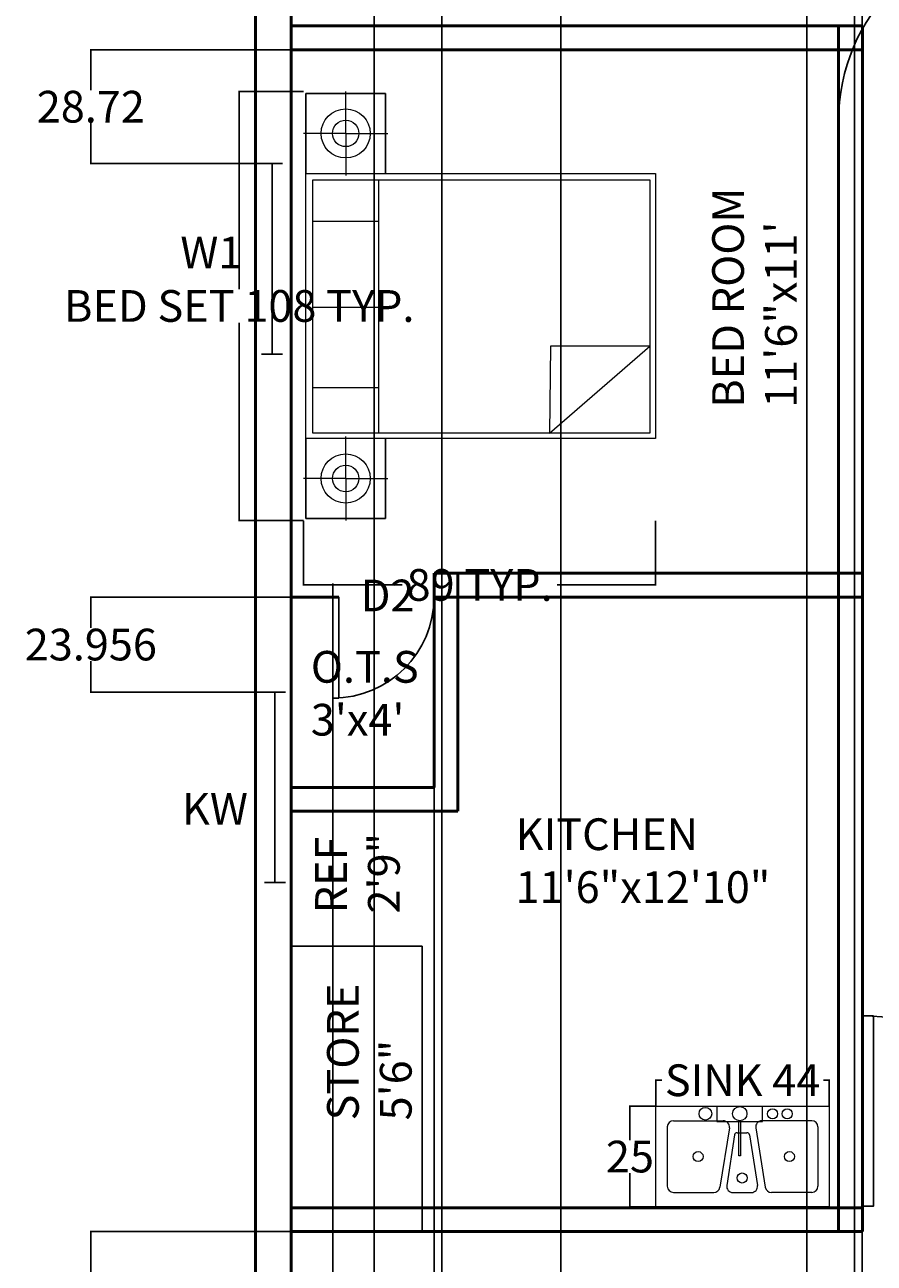
# Model space of a CAD drawing. Units: inches. Extents: x 3004 to 3478, y -798 to 114.
# Tile 3 of 5: x 3004 to 3218, y -503 to -190. Entities that reach past the tile are written whole.
import ezdxf

# ---------------------------------------------------------------- set-up
doc = ezdxf.new("R2010")
doc.units = ezdxf.units.IN
doc.header["$MEASUREMENT"] = 0
for name, color, linetype, lineweight in [('A-ANNO-DIMS', 2, 'Continuous', 18), ('A-ANNO-TEXT', 7, 'Continuous', 18), ('A-AREA-IDEN', 7, 'Continuous', 18), ('A-DOOR', 4, 'Continuous', 25), ('A-FLOR-CASE', 8, 'Continuous', 25), ('A-FLOR-FIXT', 9, 'Continuous', 18), ('A-FURN', 8, 'Continuous', 18), ('A-GLAZ', 4, 'Continuous', 25), ('A-WALL', 7, 'Continuous', 50)]:
    doc.layers.add(name, color=color, linetype=linetype, lineweight=lineweight)
doc.styles.get("Standard").update_dxf_attribs({"font": 'arial.ttf', "height": 8})
doc.dimstyles.get("Standard").update_dxf_attribs({"dimtxt": 0.18, "dimasz": 0.18, "dimexe": 0.18, "dimexo": 0.0625, "dimgap": 0.09, "dimtad": 0, "dimtih": 1, "dimtoh": 1, "dimzin": 0, "dimdsep": 46, "dimlunit": 4, "dimtxsty": 'Standard', "dimcen": 0.09, "dimadec": 0, "dimazin": 0, "dimtfac": 1, "dimtofl": 0, "dimtmove": 0, "dimatfit": 3, "dimfxl": 1, "dimtolj": 1, "dimtzin": 0, "dimarcsym": 0})

# ---------------------------------------------------------------- blocks, each defined once
blk = doc.blocks.new('A$C27EB6A15')
for p, q in [((0, 0), (0, 644.7)), ((0, 644.7), (1110.1, 644.7)), ((682.1, 643.4), (390.6, 643.4)), ((390.6, 643.4), (390.6, 547.6)), ((682.1, 547.6), (682.1, 643.4)), ((1110.1, 644.7), (1110.1, 0)), ((72.5, 512.3), (72.5, 132)), ((111.7, 551.5), (431.6, 551.5)), ((390.6, 547.6), (682.1, 547.6)), ((470.2, 506.2), (409.5, 125.9)), ((530.7, 328), (530.7, 553.3)), ((541.9, 552.9), (541.9, 328)), ((639.9, 506.2), (700.6, 125.9)), ((998.4, 551.5), (678.5, 551.5)), ((1037.5, 512.3), (1037.5, 132)), ((504.1, 462.2), (453.4, 137.6)), ((519.5, 475.4), (583.2, 475.4)), ((598.6, 462.2), (650.4, 137.8)), ((541.9, 328), (530.7, 328)), ((111.7, 92.9), (370.9, 92.9)), ((492.1, 92.5), (611.7, 92.5)), ((998.4, 92.9), (739.2, 92.9)), ((1110.1, 0), (0, 0))]:
    blk.add_line(p, q)
for centre, radius in [((317, 596.6), 40.3), ((537.2, 597.3), 45.9), ((747.1, 596.6), 32.3), ((841.3, 596.6), 32.3), ((269.9, 322.4), 32.3), ((854.7, 322.4), 32.3), ((552.2, 185.3), 32.3)]:
    blk.add_circle(centre, radius)
for centre, radius, start, end in [((111.7, 512.3), 39.1, 90, 180), ((431.6, 512.3), 39.1, 350.93428, 90), ((538.2, 591.7), 39.2, 259.3674, 275.24456), ((678.5, 512.3), 39.1, 90, 189.06572), ((998.4, 512.3), 39.1, 0, 90), ((519.5, 459.7), 15.7, 90, 171.13117), ((583.2, 459.7), 15.7, 9.06572, 90), ((111.7, 132), 39.1, 180, 270), ((370.9, 132), 39.1, 270, 350.93428), ((492.1, 131.6), 39.1, 171.13117, 270), ((611.7, 131.6), 39.1, 270, 9.06572), ((739.2, 132), 39.1, 189.06572, 270), ((998.4, 132), 39.1, 270, 0)]:
    blk.add_arc(centre, radius, start, end)
blk = doc.blocks.new('A$C214F6537')
for p, q in [((0.4648, 1.98, -0.1688), (0.0108, 1.98, -0.1688)), ((0.0108, 1.98, -0.1688), (0.0108, 1.53, -0.1688)), ((0.0108, 1.98, -0.1688), (2.4188, 1.98, -0.1688)), ((0.0108, 1.53, -0.1688), (0.0108, 1.98, -0.1688)), ((0.2381, 1.7553, -0.4388), (0.2381, 1.9934, -0.4388)), ((0.4648, 0, -0.1688), (0.4648, 1.98, -0.1688)), ((0.4648, 1.98, -0.1688), (1.9648, 1.98, -0.1688)), ((0.4648, 1.53, -0.1688), (0.4648, 1.98, -0.1688)), ((1.9648, 1.98, -0.1688), (1.9648, 0, -0.1688)), ((2.4188, 1.98, -0.1688), (1.9648, 1.98, -0.1688)), ((1.9648, 1.98, -0.1688), (1.9648, 1.53, -0.1688)), ((2.1921, 1.7553, -0.4388), (2.1921, 1.9934, -0.4388)), ((2.4188, 1.53, -0.1688), (2.4188, 1.98, -0.1688)), ((2.4188, 1.98, -0.1688), (2.4188, 1.53, -0.1688)), ((0.4951, 1.9415, -0.1688), (1.9289, 1.9415, -0.1688)), ((0.4951, 1.5702, -0.1688), (0.4951, 1.9415, -0.1688)), ((0.7525, 1.9415, -0.1688), (0.7525, 1.5702, -0.1688)), ((1.2089, 1.9415, -0.1688), (1.2089, 1.5702, -0.1688)), ((1.6942, 1.9415, -0.1688), (1.6942, 1.5702, -0.1688)), ((1.9289, 1.9415, -0.1688), (1.9289, 1.5702, -0.1688)), ((0.2381, 1.7553, -0.4388), (0, 1.7553, -0.4388)), ((0.2381, 1.7553, -0.4388), (0.2381, 1.5173, -0.4388)), ((0.2381, 1.7553, -0.4388), (0.4762, 1.7553, -0.4388)), ((2.1921, 1.7553, -0.4388), (1.954, 1.7553, -0.4388)), ((2.1921, 1.7553, -0.4388), (2.4302, 1.7553, -0.4388)), ((2.1921, 1.7553, -0.4388), (2.1921, 1.5173, -0.4388)), ((0.4951, 0.0322, -0.1688), (0.4951, 1.5702, -0.1688)), ((1.9289, 1.5702, -0.1688), (0.4951, 1.5702, -0.1688)), ((1.9289, 1.5702, -0.1688), (1.9289, 0.0322, -0.1688)), ((0.0108, 1.53, -0.1688), (0.4648, 1.53, -0.1688)), ((0.4648, 1.53, -0.1688), (0.0108, 1.53, -0.1688)), ((0.4648, 0, -0.1688), (0.4648, 1.53, -0.1688)), ((1.9648, 1.53, -0.1688), (2.4188, 1.53, -0.1688)), ((2.4188, 1.53, -0.1688), (1.9648, 1.53, -0.1688)), ((1.9648, 1.53, -0.1688), (1.9648, 0, -0.1688)), ((0.4951, 0.6005, -0.1688), (0.9872, 0.0322, -0.1688)), ((0.9872, 0.5947, -0.1688), (0.4951, 0.6005, -0.1688)), ((0.9872, 0.0322, -0.1688), (0.9872, 0.5947, -0.1688)), ((1.9648, 0, -0.1688), (0.4648, 0, -0.1688)), ((1.9648, 0, -0.1688), (0.4648, 0, -0.1688)), ((1.9289, 0.0322, -0.1688), (0.4951, 0.0322, -0.1688))]:
    blk.add_line(p, q)
for centre, radius in [((0.2381, 1.7553, -0.4388), 0.139), ((2.1921, 1.7553, -0.4388), 0.139), ((0.2381, 1.7553, -0.4388), 0.075), ((2.1921, 1.7553, -0.4388), 0.075)]:
    blk.add_circle(centre, radius)
blk = doc.blocks.new('*U17')
for p, q in [((-750, 0), (-750, -100)), ((0, 0), (0, -100))]:
    blk.add_line(p, q)
blk.add_lwpolyline([(0, 0), (0, 750), (-43.75, 750), (-43.75, 0)], close=True)
blk.add_arc((0, 0), 750, 90, 180)
blk = doc.blocks.new('*U18')
for p, q in [((0, 0), (0, 100)), ((750, 0), (750, 100))]:
    blk.add_line(p, q)
blk.add_lwpolyline([(0, 0), (0, -750), (43.75, -750), (43.75, 0)], close=True)
blk.add_arc((0, 0), 750, 270, 0)
blk = doc.blocks.new('*U16')
for p, q in [((0, 0), (0, -100)), ((750, 0), (750, -100))]:
    blk.add_line(p, q)
blk.add_lwpolyline([(0, 0), (0, 750), (43.75, 750), (43.75, 0)], close=True)
blk.add_arc((0, 0), 750, 0, 90)
blk = doc.blocks.new('Window - Imperial')
for p, q in [((0, 4), (0, 0)), ((36, 4), (36, 0)), ((0, 2), (36, 2))]:
    blk.add_line(p, q)
blk = doc.blocks.new('*D24')
at = {"layer": 'A-ANNO-DIMS', "color": 0, "lineweight": -2, "transparency": 16777216}
for p, q in [((3074.26, -207.17), (3057.91, -207.17)), ((3058.09, -207.35), (3058.09, -257.05)), ((3058.09, -315.21), (3058.09, -265.5)), ((3074.26, -315.39), (3057.91, -315.39))]:
    blk.add_line(p, q, dxfattribs=at)
at = {"layer": 'A-ANNO-DIMS', "color": 0, "transparency": 16777216}
for points in [[(3058.06, -207.35), (3058.12, -207.35), (3058.09, -207.17)], [(3058.06, -315.21), (3058.12, -315.21), (3058.09, -315.39)]]:
    blk.add_solid(points, dxfattribs=at)
at = {"layer": 'Defpoints', "color": 0, "transparency": 16777216}
for p in [(3058.09, -207.17), (3074.32, -207.17), (3074.32, -315.39)]:
    blk.add_point(p, dxfattribs=at)
at = {"layer": 'A-ANNO-DIMS', "color": 0, "transparency": 16777216, "insert": (3058.09, -261.28), "char_height": 8, "attachment_point": 5}
blk.add_mtext('\\A1;BED SET 108 TYP.', dxfattribs=at)
blk = doc.blocks.new('*D25')
at = {"layer": 'A-ANNO-DIMS', "color": 0, "lineweight": -2, "transparency": 16777216}
for p, q in [((3074.32, -315.45), (3074.32, -331.8)), ((3163.09, -315.45), (3163.09, -331.8)), ((3074.5, -331.62), (3099.14, -331.62)), ((3162.91, -331.62), (3138.27, -331.62))]:
    blk.add_line(p, q, dxfattribs=at)
at = {"layer": 'A-ANNO-DIMS', "color": 0, "transparency": 16777216}
for points in [[(3074.5, -331.59), (3074.5, -331.65), (3074.32, -331.62)], [(3162.91, -331.59), (3162.91, -331.65), (3163.09, -331.62)]]:
    blk.add_solid(points, dxfattribs=at)
at = {"layer": 'Defpoints', "color": 0, "transparency": 16777216}
for p in [(3074.32, -315.39), (3163.09, -315.39), (3074.32, -331.62)]:
    blk.add_point(p, dxfattribs=at)
at = {"layer": 'A-ANNO-DIMS', "color": 0, "transparency": 16777216, "insert": (3118.7, -331.62), "char_height": 8, "attachment_point": 5}
blk.add_mtext('\\A1;89 TYP.', dxfattribs=at)
blk = doc.blocks.new('*D30')
at = {"layer": 'A-ANNO-DIMS', "color": 0, "lineweight": -2, "transparency": 16777216}
for p, q in [((3163.16, -463.02), (3163.16, -456.34)), ((3163.34, -456.52), (3164.64, -456.52)), ((3206.69, -456.52), (3205.4, -456.52)), ((3206.87, -463.02), (3206.87, -456.34))]:
    blk.add_line(p, q, dxfattribs=at)
at = {"layer": 'A-ANNO-DIMS', "color": 0, "transparency": 16777216}
for points in [[(3163.34, -456.49), (3163.34, -456.55), (3163.16, -456.52)], [(3206.69, -456.49), (3206.69, -456.55), (3206.87, -456.52)]]:
    blk.add_solid(points, dxfattribs=at)
at = {"layer": 'Defpoints', "color": 0, "transparency": 16777216}
for p in [(3206.87, -456.52), (3163.16, -463.08), (3206.87, -463.08)]:
    blk.add_point(p, dxfattribs=at)
at = {"layer": 'A-ANNO-DIMS', "color": 0, "transparency": 16777216, "insert": (3185.02, -456.52), "char_height": 8, "attachment_point": 5}
blk.add_mtext('\\A1;SINK 44', dxfattribs=at)
blk = doc.blocks.new('*D31')
at = {"layer": 'A-ANNO-DIMS', "color": 0, "lineweight": -2, "transparency": 16777216}
for p, q in [((3163.1, -463.08), (3156.43, -463.08)), ((3156.61, -463.26), (3156.61, -471.6)), ((3156.61, -488.28), (3156.61, -479.95)), ((3163.1, -488.46), (3156.43, -488.46))]:
    blk.add_line(p, q, dxfattribs=at)
at = {"layer": 'A-ANNO-DIMS', "color": 0, "transparency": 16777216}
for points in [[(3156.58, -463.26), (3156.64, -463.26), (3156.61, -463.08)], [(3156.58, -488.28), (3156.64, -488.28), (3156.61, -488.46)]]:
    blk.add_solid(points, dxfattribs=at)
at = {"layer": 'Defpoints', "color": 0, "transparency": 16777216}
for p in [(3156.61, -463.08), (3163.16, -463.08), (3163.16, -488.46)]:
    blk.add_point(p, dxfattribs=at)
at = {"layer": 'A-ANNO-DIMS', "color": 0, "transparency": 16777216, "insert": (3156.61, -475.77), "char_height": 8, "attachment_point": 5}
blk.add_mtext('\\A1;25', dxfattribs=at)
blk = doc.blocks.new('*D50')
at = {"layer": 'A-ANNO-DIMS', "color": 0, "lineweight": -2, "transparency": 16777216}
for p, q in [((3071.15, -196.68), (3020.48, -196.68)), ((3020.66, -196.86), (3020.66, -206.86)), ((3020.66, -225.22), (3020.66, -215.21)), ((3063.64, -225.4), (3020.48, -225.4))]:
    blk.add_line(p, q, dxfattribs=at)
at = {"layer": 'A-ANNO-DIMS', "color": 0, "transparency": 16777216}
for points in [[(3020.63, -196.86), (3020.69, -196.86), (3020.66, -196.68)], [(3020.63, -225.22), (3020.69, -225.22), (3020.66, -225.4)]]:
    blk.add_solid(points, dxfattribs=at)
at = {"layer": 'Defpoints', "color": 0, "transparency": 16777216}
for p in [(3071.21, -196.68), (3020.66, -225.4), (3063.7, -225.4)]:
    blk.add_point(p, dxfattribs=at)
at = {"layer": 'A-ANNO-DIMS', "color": 0, "transparency": 16777216, "insert": (3020.66, -211.04), "char_height": 8, "attachment_point": 5}
blk.add_mtext('\\A1;28.72', dxfattribs=at)
blk = doc.blocks.new('*D51')
at = {"layer": 'A-ANNO-DIMS', "color": 0, "lineweight": -2, "transparency": 16777216}
for p, q in [((3071.15, -334.68), (3020.48, -334.68)), ((3020.66, -334.86), (3020.66, -342.48)), ((3020.66, -358.45), (3020.66, -350.83)), ((3064.37, -358.63), (3020.48, -358.63))]:
    blk.add_line(p, q, dxfattribs=at)
at = {"layer": 'A-ANNO-DIMS', "color": 0, "transparency": 16777216}
for points in [[(3020.63, -334.86), (3020.69, -334.86), (3020.66, -334.68)], [(3020.63, -358.45), (3020.69, -358.45), (3020.66, -358.63)]]:
    blk.add_solid(points, dxfattribs=at)
at = {"layer": 'Defpoints', "color": 0, "transparency": 16777216}
for p in [(3071.21, -334.68), (3020.66, -358.63), (3064.43, -358.63)]:
    blk.add_point(p, dxfattribs=at)
at = {"layer": 'A-ANNO-DIMS', "color": 0, "transparency": 16777216, "insert": (3020.66, -346.66), "char_height": 8, "attachment_point": 5}
blk.add_mtext('\\A1;23.956', dxfattribs=at)
blk = doc.blocks.new('*D52')
at = {"layer": 'A-ANNO-DIMS', "color": 0, "lineweight": -2, "transparency": 16777216}
for p, q in [((3071.15, -494.68), (3020.48, -494.68)), ((3020.66, -494.86), (3020.66, -517.2)), ((3020.66, -547.9), (3020.66, -525.56)), ((3064.06, -548.08), (3020.48, -548.08))]:
    blk.add_line(p, q, dxfattribs=at)
at = {"layer": 'A-ANNO-DIMS', "color": 0, "transparency": 16777216}
for points in [[(3020.63, -494.86), (3020.69, -494.86), (3020.66, -494.68)], [(3020.63, -547.9), (3020.69, -547.9), (3020.66, -548.08)]]:
    blk.add_solid(points, dxfattribs=at)
at = {"layer": 'Defpoints', "color": 0, "transparency": 16777216}
for p in [(3071.21, -494.68), (3020.66, -548.08), (3064.12, -548.08)]:
    blk.add_point(p, dxfattribs=at)
at = {"layer": 'A-ANNO-DIMS', "color": 0, "transparency": 16777216, "insert": (3020.66, -521.38), "char_height": 8, "attachment_point": 5}
blk.add_mtext('\\A1;53.4', dxfattribs=at)
blk = doc.blocks.new('*D53')
at = {"layer": 'A-ANNO-DIMS', "color": 0, "lineweight": -2, "transparency": 16777216}
for p, q in [((3092.13, 11.22), (3092.13, -793.41)), ((3071.21, 7.26), (3071.21, -793.41)), ((3071.39, -793.23), (3091.95, -793.23)), ((3092.13, -793.23), (3092.31, -793.23))]:
    blk.add_line(p, q, dxfattribs=at)
at = {"layer": 'A-ANNO-DIMS', "color": 0, "transparency": 16777216}
for points in [[(3071.39, -793.2), (3071.39, -793.26), (3071.21, -793.23)], [(3091.95, -793.2), (3091.95, -793.26), (3092.13, -793.23)]]:
    blk.add_solid(points, dxfattribs=at)
at = {"layer": 'Defpoints', "color": 0, "transparency": 16777216}
for p in [(3092.13, 11.28), (3071.21, 7.32), (3092.13, -793.23)]:
    blk.add_point(p, dxfattribs=at)
at = {"layer": 'A-ANNO-DIMS', "color": 0, "transparency": 16777216, "insert": (3105.93, -793.23), "char_height": 8, "attachment_point": 5}
blk.add_mtext('\\A1;20.92', dxfattribs=at)
blk = doc.blocks.new('*D55')
at = {"layer": 'A-ANNO-DIMS', "color": 0, "lineweight": -2, "transparency": 16777216}
for p, q in [((3215.21, -494.62), (3215.21, 109.05)), ((3215.39, 108.87), (3233.22, 108.87)), ((3263.03, 108.87), (3245.2, 108.87)), ((3263.21, -494.62), (3263.21, 109.05))]:
    blk.add_line(p, q, dxfattribs=at)
at = {"layer": 'A-ANNO-DIMS', "color": 0, "transparency": 16777216}
for points in [[(3215.39, 108.9), (3215.39, 108.84), (3215.21, 108.87)], [(3263.03, 108.9), (3263.03, 108.84), (3263.21, 108.87)]]:
    blk.add_solid(points, dxfattribs=at)
at = {"layer": 'Defpoints', "color": 0, "transparency": 16777216}
for p in [(3263.21, 108.87), (3215.21, -494.68), (3263.21, -494.68)]:
    blk.add_point(p, dxfattribs=at)
at = {"layer": 'A-ANNO-DIMS', "color": 0, "transparency": 16777216, "insert": (3239.21, 108.87), "char_height": 8, "attachment_point": 5}
blk.add_mtext('\\A1;48', dxfattribs=at)
blk = doc.blocks.new('*D57')
at = {"layer": 'A-ANNO-DIMS', "color": 0, "lineweight": -2, "transparency": 16777216}
for p, q in [((3201.21, -644.62), (3201.21, 109.05)), ((3201.39, 108.87), (3201.81, 108.87)), ((3213.03, 108.87), (3212.61, 108.87)), ((3213.21, -644.62), (3213.21, 109.05))]:
    blk.add_line(p, q, dxfattribs=at)
at = {"layer": 'A-ANNO-DIMS', "color": 0, "transparency": 16777216}
for points in [[(3201.39, 108.9), (3201.39, 108.84), (3201.21, 108.87)], [(3213.03, 108.9), (3213.03, 108.84), (3213.21, 108.87)]]:
    blk.add_solid(points, dxfattribs=at)
at = {"layer": 'Defpoints', "color": 0, "transparency": 16777216}
for p in [(3213.21, 108.87), (3201.21, -644.68), (3213.21, -644.68)]:
    blk.add_point(p, dxfattribs=at)
at = {"layer": 'A-ANNO-DIMS', "color": 0, "transparency": 16777216, "insert": (3207.21, 108.87), "char_height": 8, "attachment_point": 5}
blk.add_mtext('\\A1;12', dxfattribs=at)
blk = doc.blocks.new('*D62')
at = {"layer": 'A-ANNO-DIMS', "color": 0, "lineweight": -2, "transparency": 16777216}
for p, q in [((3081.71, -334.74), (3081.71, -793.41)), ((3107.21, -334.74), (3107.21, -793.41)), ((3081.89, -793.23), (3083.88, -793.23)), ((3107.03, -793.23), (3105.04, -793.23))]:
    blk.add_line(p, q, dxfattribs=at)
at = {"layer": 'A-ANNO-DIMS', "color": 0, "transparency": 16777216}
for points in [[(3081.89, -793.2), (3081.89, -793.26), (3081.71, -793.23)], [(3107.03, -793.2), (3107.03, -793.26), (3107.21, -793.23)]]:
    blk.add_solid(points, dxfattribs=at)
at = {"layer": 'Defpoints', "color": 0, "transparency": 16777216}
for p in [(3081.71, -334.68), (3107.21, -334.68), (3107.21, -793.23)]:
    blk.add_point(p, dxfattribs=at)
at = {"layer": 'A-ANNO-DIMS', "color": 0, "transparency": 16777216, "insert": (3094.46, -793.23), "char_height": 8, "attachment_point": 5}
blk.add_mtext('\\A1;25.5', dxfattribs=at)
blk = doc.blocks.new('*D64')
at = {"layer": 'A-ANNO-DIMS', "color": 0, "lineweight": -2, "transparency": 16777216}
for p, q in [((3215.21, -190.74), (3215.21, -793.41)), ((3257.21, -220.74), (3257.21, -793.41)), ((3215.39, -793.23), (3230.27, -793.23)), ((3257.03, -793.23), (3242.15, -793.23))]:
    blk.add_line(p, q, dxfattribs=at)
at = {"layer": 'A-ANNO-DIMS', "color": 0, "transparency": 16777216}
for points in [[(3215.39, -793.2), (3215.39, -793.26), (3215.21, -793.23)], [(3257.03, -793.2), (3257.03, -793.26), (3257.21, -793.23)]]:
    blk.add_solid(points, dxfattribs=at)
at = {"layer": 'Defpoints', "color": 0, "transparency": 16777216}
for p in [(3215.21, -190.68), (3257.21, -220.68), (3257.21, -793.23)]:
    blk.add_point(p, dxfattribs=at)
at = {"layer": 'A-ANNO-DIMS', "color": 0, "transparency": 16777216, "insert": (3236.21, -793.23), "char_height": 8, "attachment_point": 5}
blk.add_mtext('\\A1;42', dxfattribs=at)
blk = doc.blocks.new('*D65')
at = {"layer": 'A-ANNO-DIMS', "color": 0, "lineweight": -2, "transparency": 16777216}
for p, q in [((3109.21, -46.74), (3109.21, -793.41)), ((3139.21, -46.74), (3139.21, -793.41)), ((3109.39, -793.23), (3118.41, -793.23)), ((3139.03, -793.23), (3130.01, -793.23))]:
    blk.add_line(p, q, dxfattribs=at)
at = {"layer": 'A-ANNO-DIMS', "color": 0, "transparency": 16777216}
for points in [[(3109.39, -793.2), (3109.39, -793.26), (3109.21, -793.23)], [(3139.03, -793.2), (3139.03, -793.26), (3139.21, -793.23)]]:
    blk.add_solid(points, dxfattribs=at)
at = {"layer": 'Defpoints', "color": 0, "transparency": 16777216}
for p in [(3109.21, -46.68), (3139.21, -46.68), (3139.21, -793.23)]:
    blk.add_point(p, dxfattribs=at)
at = {"layer": 'A-ANNO-DIMS', "color": 0, "transparency": 16777216, "insert": (3124.21, -793.23), "char_height": 8, "attachment_point": 5}
blk.add_mtext('\\A1;30', dxfattribs=at)

msp = doc.modelspace()

# ---------------------------------------------------------------- linework, layer by layer
at = {"layer": 'A-FLOR-CASE'}
for q in [(3071.2113, -422.6779), (3104.2113, -494.6779)]:
    msp.add_line((3104.2113, -422.6779), q, dxfattribs=at)
at = {"layer": 'A-WALL'}
for p, q in [((3062.2113, 16.3221), (3062.2113, -703.6779)), ((3071.2113, 7.3221), (3071.2113, -703.6779)), ((3215.2113, -190.6779), (3071.2113, -190.6779)), ((3209.2113, -190.6779), (3209.2113, -494.6779)), ((3215.2113, -190.6779), (3215.2113, -494.6779)), ((3215.2113, -196.6779), (3071.2113, -196.6779)), ((3215.2113, -328.6779), (3107.2113, -328.6779)), ((3107.2113, -328.6779), (3107.2113, -382.6779)), ((3113.2113, -328.6779), (3113.2113, -388.6779)), ((3083.2113, -334.6779), (3071.2113, -334.6779)), ((3215.2113, -334.6779), (3107.2113, -334.6779)), ((3107.2113, -382.6779), (3071.2113, -382.6779)), ((3113.2113, -388.6779), (3071.2113, -388.6779)), ((3215.2113, -488.6779), (3071.2113, -488.6779)), ((3215.2113, -494.6779), (3071.2113, -494.6779))]:
    msp.add_line(p, q, dxfattribs=at)

# ---------------------------------------------------------------- block references
at = {"layer": 'A-DOOR'}
for name, p, xscale, yscale, zscale in [('*U17', (3257.2113, -214.6779), 0.0639999999999998, 0.0639999999999998, 0.0639999999999998), ('*U18', (3081.7115, -334.6779), 0.0339823008849558, 0.0339823008849558, 0.0339823008849558), ('*U16', (3215.2113, -488.2779), 0.0640000000000003, 0.0640000000000003, 0.0640000000000003)]:
    msp.add_blockref(name, p, dxfattribs=dict(at, xscale=xscale, yscale=yscale, zscale=zscale))
at = {"layer": 'A-FLOR-FIXT', "xscale": 0.0393700787401575, "yscale": 0.0393700787401575, "zscale": 0.0393700787401575}
msp.add_blockref('A$C27EB6A15', (3163.1638, -488.4634), dxfattribs=at)
at = {"layer": 'A-FURN', "xscale": 44.53130442995502, "yscale": 44.53130442995502, "zscale": 44.53130442995502, "rotation": 89.99999999999999}
msp.add_blockref('A$C214F6537', (3163.0893, -315.3851, 7.5147), dxfattribs=at)
at = {"layer": 'A-GLAZ', "xscale": 1.333333333333333, "yscale": 1.333333333333333, "zscale": 1.333333333333333, "rotation": 270}
for p in [(3063.6984, -225.3967), (3064.4315, -358.6343)]:
    msp.add_blockref('Window - Imperial', p, dxfattribs=at)

# ---------------------------------------------------------------- texts
at = {"layer": 'A-ANNO-TEXT', "char_height": 8, "attachment_point": 1}
for s, width, insert in [('W1', 86.182133, (3043.2333, -243.8174)), ('D2', 22.083935, (3088.7278, -330.2837)), ('KW', 86.182133, (3043.6383, -384.1139))]:
    msp.add_mtext_dynamic_manual_height_columns(s, width=width, gutter_width=40, heights=[0], dxfattribs=dict(at, insert=insert))
at = {"layer": 'A-AREA-IDEN', "char_height": 8, "attachment_point": 1, "rotation": 90}
for s, width, insert in [('BED ROOM\\P11\'6"x11\'', 228.23715, (3177.3501, -286.9432)), ('REF\\P2\'9"', 21.347239, (3077.2227, -414.473)), ('STORE\\P5\'6"', 22.748729, (3080.2227, -466.647))]:
    msp.add_mtext_dynamic_manual_height_columns(s, width=width, gutter_width=40, heights=[0], dxfattribs=dict(at, insert=insert))
at = {"layer": 'A-AREA-IDEN', "char_height": 8, "attachment_point": 1}
for s, width, insert in [("O.T.S\\P3'x4'", 22.748729, (3076.1356, -348.2759)), ('KITCHEN\\P11\'6"x12\'10"', 228.23715, (3127.7657, -390.4872))]:
    msp.add_mtext_dynamic_manual_height_columns(s, width=width, gutter_width=40, heights=[0], dxfattribs=dict(at, insert=insert))

# ---------------------------------------------------------------- dimensions: what is measured, and where the dimension line sits
at = {"layer": 'A-ANNO-DIMS'}
for base, p1, p2, override, picture, middle in [((3213.2113, 108.8721), (3201.2113, -644.6779), (3213.2113, -644.6779), {"dimdec": 0, "dimlfac": 1, "dimrnd": 0, "dimzin": 0, "dimdsep": 46, "dimlunit": 2}, '*D57', (3207.2113, 108.8721)), ((3263.2113, 108.8721), (3215.2113, -494.6779), (3263.2113, -494.6779), {"dimdec": 0, "dimlfac": 1, "dimrnd": 0, "dimzin": 0, "dimdsep": 46, "dimlunit": 2}, '*D55', (3239.2113, 108.8721)), ((3092.1316, -793.2279), (3071.2113, 7.3221), (3092.1316, 11.284), {"dimdec": 2, "dimlfac": 1, "dimrnd": 0, "dimzin": 0, "dimdsep": 46, "dimlunit": 2}, '*D53', (3105.9268, -793.2279)), ((3139.2113, -793.2279), (3109.2113, -46.6779), (3139.2113, -46.6779), {"dimdec": 0, "dimlfac": 1, "dimrnd": 0, "dimzin": 0, "dimdsep": 46, "dimlunit": 2}, '*D65', (3124.2113, -793.2279)), ((3257.2113, -793.2279), (3215.2113, -190.6779), (3257.2113, -220.6779), {"dimdec": 0, "dimlfac": 1, "dimrnd": 0, "dimzin": 0, "dimdsep": 46, "dimlunit": 2}, '*D64', (3236.2113, -793.2279)), ((3107.2113, -793.2279), (3081.7115, -334.6779), (3107.2113, -334.6779), {"dimdec": 1, "dimlfac": 1, "dimrnd": 0, "dimzin": 0, "dimdsep": 46, "dimlunit": 2}, '*D62', (3094.4614, -793.2279))]:
    dim = msp.add_linear_dim(base=base, p1=p1, p2=p2, dimstyle='Standard', override=override, dxfattribs=at)
    dim.commit()
    dim.dimension.update_dxf_attribs({"geometry": picture, "text_midpoint": middle})
for base, p1, p2, override, picture, middle in [((3020.6613, -225.3967), (3071.2113, -196.6779), (3063.6984, -225.3967), {"dimdec": 2, "dimlfac": 1, "dimrnd": 0, "dimzin": 0, "dimdsep": 46, "dimlunit": 2}, '*D50', (3020.6613, -211.0373)), ((3020.6613, -358.6343), (3071.2113, -334.6779), (3064.4315, -358.6343), {"dimdec": 3, "dimlfac": 1, "dimrnd": 0, "dimzin": 0, "dimdsep": 46, "dimlunit": 2}, '*D51', (3020.6613, -346.6561)), ((3156.6082, -463.0804), (3163.1638, -488.4634), (3163.1638, -463.0804), {"dimdec": 0, "dimlfac": 1, "dimrnd": 0, "dimzin": 0, "dimdsep": 46, "dimlunit": 2}, '*D31', (3156.6082, -475.7719)), ((3020.6613, -548.0828), (3071.2113, -494.6779), (3064.1176, -548.0828), {"dimdec": 1, "dimlfac": 1, "dimrnd": 0, "dimzin": 0, "dimdsep": 46, "dimlunit": 2}, '*D52', (3020.6613, -521.3803))]:
    dim = msp.add_linear_dim(base=base, p1=p1, p2=p2, angle=90, dimstyle='Standard', override=override, dxfattribs=at)
    dim.commit()
    dim.dimension.update_dxf_attribs({"geometry": picture, "text_midpoint": middle})
for base, p1, p2, angle, text, picture, middle in [((3058.086, -207.1659), (3074.3189, -315.3851), (3074.3189, -207.1659), 90, 'BED SET <> TYP.', '*D24', (3058.086, -261.2755)), ((3074.3189, -331.618), (3163.0893, -315.3851), (3074.3189, -315.3851), 180, '<> TYP.', '*D25', (3118.7041, -331.618))]:
    dim = msp.add_linear_dim(base=base, p1=p1, p2=p2, angle=angle, text=text, dimstyle='Standard', override={"dimdec": 0, "dimlfac": 1, "dimrnd": 0, "dimzin": 0, "dimdsep": 46, "dimlunit": 2}, dxfattribs=at)
    dim.commit()
    dim.dimension.update_dxf_attribs({"geometry": picture, "text_midpoint": middle})
dim = msp.add_linear_dim(base=(3206.8682, -456.5247), p1=(3163.1638, -463.0804), p2=(3206.8682, -463.0804), text='SINK <>', dimstyle='Standard', override={"dimdec": 0, "dimlfac": 1, "dimrnd": 0, "dimzin": 0, "dimdsep": 46, "dimlunit": 2}, dxfattribs=at)
dim.commit()
dim.dimension.update_dxf_attribs({"geometry": '*D30', "text_midpoint": (3185.016, -456.5247)})

doc.saveas('drawing.dxf')
